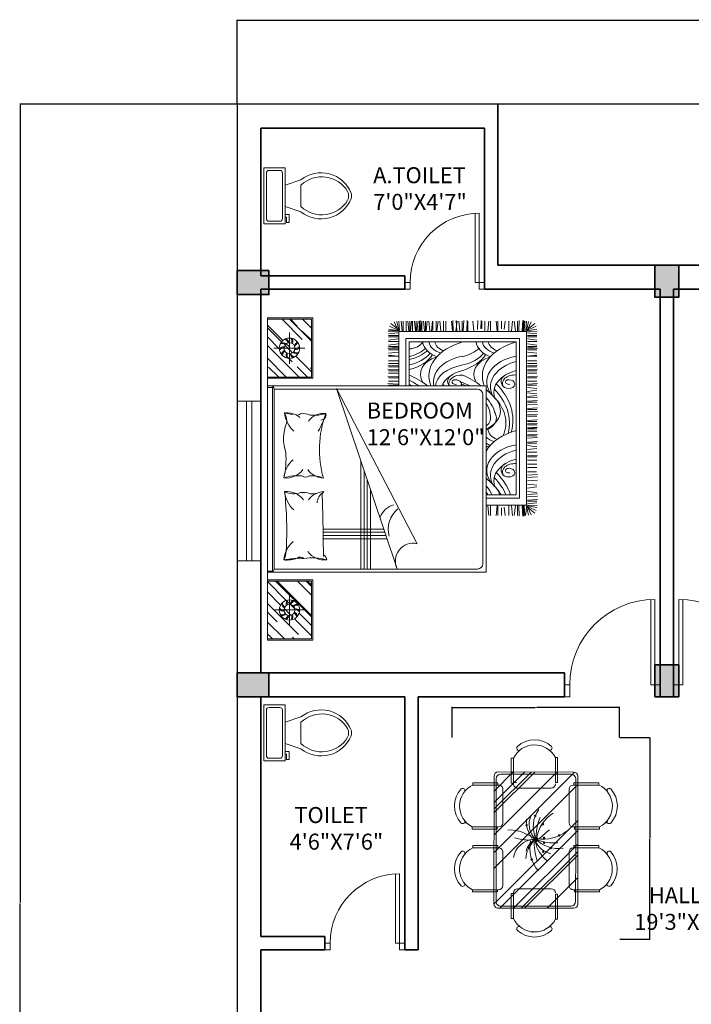
# Model space of a CAD drawing. Units: inches. Extents: x 1602 to 2642, y 1463 to 2270.
# Tile 2 of 5: x 1602 to 1854, y 1763 to 2132. Entities that reach past the tile are written whole.
import ezdxf

# ---------------------------------------------------------------- set-up
doc = ezdxf.new("R2010")
doc.units = ezdxf.units.IN
for name, color, linetype, lineweight in [('A-ANNO-DIMS', 2, 'Continuous', 18), ('A-AREA-IDEN', 7, 'Continuous', 18), ('A-COLS', 7, 'Continuous', 35), ('A-DOOR', 3, 'Continuous', 18), ('A-FLOR-FIXT', 8, 'Continuous', 18), ('A-FURN', 8, 'Continuous', 13), ('A-GLAZ', 4, 'Continuous', 18), ('A-WALL', 7, 'Continuous', 35), ('C-PROP', 7, 'Continuous', 25)]:
    doc.layers.add(name, color=color, linetype=linetype, lineweight=lineweight)
doc.styles.get("Standard").update_dxf_attribs({"font": 'arial.ttf'})
doc.dimstyles.get("Standard").update_dxf_attribs({"dimtxt": 0.18, "dimasz": 0.18, "dimexe": 0.18, "dimexo": 0.0625, "dimgap": 0.09, "dimtad": 0, "dimtih": 1, "dimtoh": 1, "dimdec": 4, "dimzin": 0, "dimdsep": 46, "dimtxsty": 'Standard', "dimcen": 0.09, "dimadec": 0, "dimazin": 0, "dimtfac": 1, "dimtdec": 4, "dimtofl": 0, "dimtmove": 0, "dimatfit": 3, "dimfxl": 1, "dimtolj": 1, "dimtzin": 0, "dimarcsym": 0})

# ---------------------------------------------------------------- blocks, each defined once
blk = doc.blocks.new('*U3')
for p, q in [((9.5, -6), (9.5, -2)), ((-10, -8.5), (-8, -8.5)), ((-10, -9.5), (-10, -8.5)), ((-7, -9.5), (-10, -9.5)), ((-8, -8.5), (-8, -8)), ((-7, -8), (-7, -9.5)), ((-4, -8), (-6, -14)), ((4, -8), (6, -14)), ((4, -14), (-4, -14))]:
    blk.add_line(p, q)
blk.add_lwpolyline([(10.5, -8), (10.5, 0), (-10.5, 0), (-10.5, -8)], close=True)
for points in [[(-9.5, -2), (-9.5, -6)], [(8.5, -1), (-8.5, -1)], [(-8.5, -7), (8.5, -7)]]:
    blk.add_lwpolyline(points)
for centre, radius, start, end in [((-8.62, -1.88), 0.884, 81.8699, 188.1301), ((8.62, -1.88), 0.884, 351.8699, 98.1301), ((-8.62, -6.12), 0.884, 171.8699, 278.1301), ((8.62, -6.12), 0.884, 261.8699, 8.1301), ((3.52, -21.58), 12.17, 141.4691, 247.9714), ((4.2, -21.82), 11.33, 136.3677, 238.9468), ((-3.52, -21.58), 12.17, 292.0284, 38.5307), ((-4.2, -21.82), 11.33, 301.053, 43.6321), ((0, -27.88), 4, 245.7318, 294.2682), ((0, -29), 4, 254.8605, 285.1395)]:
    blk.add_arc(centre, radius, start, end)
blk = doc.blocks.new('A$C6327331B')
for p, q in [((790.8, 678.3), (790.8, 696.4)), ((790.8, 678.3), (790.8, 696.4)), ((1381.3, 692.8), (1381.3, 686.2)), ((1381.3, 692.8), (1381.3, 686.2)), ((410.1, 615.8), (410, 377)), ((410.1, 615.8), (410, 377)), ((431.6, 615.8), (410.1, 615.8)), ((431.6, 615.8), (410.1, 615.8)), ((431.4, 376.9), (431.6, 615.8)), ((431.4, 376.9), (431.6, 615.8)), ((431.5, 571.8), (431.4, 370.8)), ((431.5, 571.8), (431.4, 370.8)), ((831.4, 382.9), (831.6, 621.7)), ((831.4, 382.9), (831.6, 621.7)), ((831.4, 370.6), (831.5, 571.6)), ((831.4, 370.6), (831.5, 571.6)), ((831.6, 621.7), (853, 621.7)), ((831.6, 621.7), (853, 621.7)), ((853, 621.7), (852.9, 382.9)), ((853, 621.7), (852.9, 382.9)), ((1009.3, 615.5), (1009.2, 376.7)), ((1009.3, 615.5), (1009.2, 376.7)), ((1030.7, 615.5), (1009.3, 615.5)), ((1030.7, 615.5), (1009.3, 615.5)), ((1030.6, 376.6), (1030.7, 615.5)), ((1030.6, 376.6), (1030.7, 615.5)), ((1030.7, 571.5), (1030.6, 370.5)), ((1030.7, 571.5), (1030.6, 370.5)), ((1430.6, 382.6), (1430.7, 621.4)), ((1430.6, 382.6), (1430.7, 621.4)), ((1430.6, 370.3), (1430.7, 571.3)), ((1430.6, 370.3), (1430.7, 571.3)), ((1430.7, 621.4), (1452.2, 621.4)), ((1430.7, 621.4), (1452.2, 621.4)), ((1452.2, 621.4), (1452, 382.6)), ((1452.2, 621.4), (1452, 382.6)), ((1075.9, -386.3), (308.5, 383.1)), ((1075.9, -386.3), (308.5, 383.1)), ((347.5, 414), (831.5, 413.8)), ((347.5, 414), (831.5, 413.8)), ((372.5, 394), (831.4, 393.8)), ((372.5, 394), (1009.2, 393.7)), ((410, 377), (431.4, 376.9)), ((410, 377), (431.4, 376.9)), ((1226.3, -386.4), (428, 414)), ((1226.3, -386.4), (428, 414)), ((1567.1, -386.6), (768.8, 413.8)), ((1567.1, -386.6), (768.8, 413.8)), ((852.9, 382.9), (831.4, 382.9)), ((852.9, 382.9), (831.4, 382.9)), ((831.5, 413.8), (1567.5, 413.4)), ((1607.1, -331.3), (864.1, 413.8)), ((1607.1, -331.3), (864.1, 413.8)), ((1607.2, -200.8), (994.4, 413.7)), ((1607.2, -200.8), (994.4, 413.7)), ((1009.2, 413.7), (1567.5, 413.4)), ((1009.2, 393.7), (1542.5, 393.4)), ((1009.2, 376.7), (1030.6, 376.6)), ((1009.2, 376.7), (1030.6, 376.6)), ((1607.2, -125.5), (1069.5, 413.7)), ((1607.2, -125.5), (1069.5, 413.7)), ((1607.2, -95.4), (1099.6, 413.6)), ((1607.2, -95.4), (1099.6, 413.6)), ((1607.3, 120.5), (1315.1, 413.5)), ((1607.3, 120.5), (1315.1, 413.5)), ((1415.7, 413.4), (1415.7, 413.5)), ((1415.7, 413.4), (1415.7, 413.5)), ((1452, 382.6), (1430.6, 382.6)), ((1452, 382.6), (1430.6, 382.6)), ((307.1, -346), (307.5, 374)), ((307.1, -346), (307.5, 374)), ((327.1, -321), (327.5, 349)), ((471.4, 330.8), (791.4, 330.6)), ((471.4, 330.8), (791.4, 330.6)), ((1070.6, 330.5), (1390.6, 330.3)), ((1070.6, 330.5), (1390.6, 330.3)), ((1587.5, 348.4), (1587.1, -321.6)), ((1607.5, 373.4), (1607.1, -346.6)), ((1607.5, 373.4), (1607.1, -346.6)), ((169.9, 221.5), (408.7, 221.6)), ((169.9, 221.5), (408.7, 221.6)), ((169.9, 200.1), (169.9, 221.5)), ((169.9, 200.1), (169.9, 221.5)), ((408.7, 200.2), (169.9, 200.1)), ((408.7, 200.2), (169.9, 200.1)), ((905.5, -386.3), (307.4, 213.5)), ((905.5, -386.3), (307.4, 213.5)), ((408.7, 221.6), (408.7, 200.2)), ((408.7, 221.6), (408.7, 200.2)), ((1473.3, 221.6), (1473.3, 200.2)), ((1473.3, 221.6), (1473.3, 200.2)), ((1712.1, 221.5), (1473.3, 221.6)), ((1712.1, 221.5), (1473.3, 221.6)), ((1473.3, 200.2), (1712.1, 200.1)), ((1473.3, 200.2), (1712.1, 200.1)), ((1712.1, 200.1), (1712.1, 221.5)), ((1712.1, 200.1), (1712.1, 221.5)), ((461.2, -159.8), (461, 160.2)), ((461.2, -159.8), (461, 160.2)), ((1420.8, -159.8), (1420.9, 160.2)), ((1420.8, -159.8), (1420.9, 160.2)), ((695.1, -386.2), (307.3, 2.7)), ((695.1, -386.2), (307.3, 2.7)), ((44.6, -20.2), (44.5, -20.1)), ((44.6, -20.2), (44.5, -20.1)), ((599.8, -386.1), (307.2, -92.7)), ((599.8, -386.1), (307.2, -92.7)), ((660, -386.1), (307.3, -32.5)), ((660, -386.1), (307.3, -32.5)), ((1837.4, -20.2), (1837.5, -20.1)), ((1837.4, -20.2), (1837.5, -20.1)), ((408.7, -193.6), (408.7, -172.1)), ((408.7, -193.6), (408.7, -172.1)), ((415.1, -199.8), (176.2, -199.9)), ((415.1, -199.8), (176.2, -199.9)), ((176.2, -199.9), (176.2, -221.3)), ((176.2, -199.9), (176.2, -221.3)), ((176.2, -221.3), (415.1, -221.2)), ((176.2, -221.3), (415.1, -221.2)), ((220.2, -199.9), (421.2, -199.8)), ((220.2, -199.9), (421.2, -199.8)), ((489.6, -386), (307.2, -203.2)), ((489.6, -386), (307.2, -203.2)), ((415.1, -221.2), (415.1, -199.8)), ((415.1, -221.2), (415.1, -199.8)), ((1661.8, -199.9), (1460.8, -199.8)), ((1661.8, -199.9), (1460.8, -199.8)), ((1466.9, -221.2), (1466.9, -199.8)), ((1466.9, -221.2), (1466.9, -199.8)), ((1466.9, -199.8), (1705.7, -199.9)), ((1466.9, -199.8), (1705.7, -199.9)), ((1705.7, -221.3), (1466.9, -221.2)), ((1705.7, -221.3), (1466.9, -221.2)), ((1705.7, -199.9), (1705.7, -221.3)), ((1705.7, -199.9), (1705.7, -221.3)), ((1542.1, -366.6), (372.1, -366)), ((410.1, -587.7), (410, -348.9)), ((410.1, -587.7), (410, -348.9)), ((410, -348.9), (431.4, -348.9)), ((410, -348.9), (431.4, -348.9)), ((431.5, -543.7), (431.4, -342.7)), ((431.5, -543.7), (431.4, -342.7)), ((431.4, -348.9), (431.6, -587.7)), ((431.4, -348.9), (431.6, -587.7)), ((471.4, -302.7), (791.4, -302.5)), ((471.4, -302.7), (791.4, -302.5)), ((831.4, -342.5), (831.5, -543.5)), ((831.4, -342.5), (831.5, -543.5)), ((831.4, -354.8), (831.6, -593.6)), ((831.4, -354.8), (831.6, -593.6)), ((852.9, -354.8), (831.4, -354.8)), ((852.9, -354.8), (831.4, -354.8)), ((853, -593.6), (852.9, -354.8)), ((853, -593.6), (852.9, -354.8)), ((1009.2, -348.6), (1030.6, -348.5)), ((1009.2, -348.6), (1030.6, -348.5)), ((1009.3, -587.4), (1009.2, -348.6)), ((1009.3, -587.4), (1009.2, -348.6)), ((1030.7, -543.4), (1030.6, -342.4)), ((1030.7, -543.4), (1030.6, -342.4)), ((1030.6, -348.5), (1030.7, -587.4)), ((1030.6, -348.5), (1030.7, -587.4)), ((1070.6, -302.4), (1390.6, -302.2)), ((1070.6, -302.4), (1390.6, -302.2)), ((1430.6, -342.2), (1430.7, -543.2)), ((1430.6, -342.2), (1430.7, -543.2)), ((1430.6, -354.5), (1430.7, -593.3)), ((1430.6, -354.5), (1430.7, -593.3)), ((1452, -354.5), (1430.6, -354.5)), ((1452, -354.5), (1430.6, -354.5)), ((1452.2, -593.3), (1452, -354.5)), ((1452.2, -593.3), (1452, -354.5)), ((1567.1, -386.6), (347.1, -386)), ((1567.1, -386.6), (347.1, -386)), ((831.5, -385.7), (864.1, -385.7)), ((831.5, -385.7), (864.1, -385.7)), ((1415.7, -385.3), (1415.7, -385.4)), ((1415.7, -385.3), (1415.7, -385.4)), ((431.6, -587.7), (410.1, -587.7)), ((431.6, -587.7), (410.1, -587.7)), ((790.8, -650.2), (790.8, -668.4)), ((790.8, -650.2), (790.8, -668.4)), ((831.6, -593.6), (853, -593.6)), ((831.6, -593.6), (853, -593.6)), ((1030.7, -587.4), (1009.3, -587.4)), ((1030.7, -587.4), (1009.3, -587.4)), ((1430.7, -593.3), (1452.2, -593.3)), ((1430.7, -593.3), (1452.2, -593.3)), ((1381.3, -664.7), (1381.3, -658.1)), ((1381.3, -664.7), (1381.3, -658.1))]:
    blk.add_line(p, q)
for centre, radius, start, end in [((631.5, 550.5), 241.3, 47.46915, 132.47205), ((631.5, 550.5), 241.3, 47.46915, 132.47205), ((1230.7, 550.2), 241.3, 47.46915, 132.47205), ((1230.7, 550.2), 241.3, 47.46915, 132.47205), ((633, 521.6), 222.4, 26.76564, 154.93691), ((633, 521.6), 222.4, 26.76564, 154.93691), ((484.3, 714.2), 21.2, 137.64965, 300.34124), ((484.3, 714.2), 21.2, 137.64965, 300.34124), ((779, 714), 21.2, 239.59996, 42.29154), ((779, 714), 21.2, 239.59996, 42.29154), ((1232.2, 521.3), 222.4, 84.42654, 154.93691), ((1232.2, 521.3), 222.4, 84.42654, 154.93691), ((1083.4, 713.9), 21.2, 137.64965, 300.34124), ((1083.4, 713.9), 21.2, 137.64965, 300.34124), ((1232.2, 521.3), 222.4, 26.76564, 84.42654), ((1232.2, 521.3), 222.4, 26.76564, 84.42654), ((1378.1, 713.7), 21.2, 239.59996, 42.29154), ((1378.1, 713.7), 21.2, 239.59996, 42.29154), ((347.5, 374), 40, 89.9706, 179.9706), ((347.5, 374), 40, 89.9706, 179.9706), ((372.5, 349), 45, 89.9706, 179.9706), ((1542.5, 348.4), 45, 359.9706, 89.9706), ((1567.5, 373.4), 40, 359.9706, 89.9706), ((1567.5, 373.4), 40, 359.9706, 89.9706), ((471.4, 370.8), 40, 179.9706, 269.9706), ((471.4, 370.8), 40, 179.9706, 269.9706), ((791.4, 370.6), 40, 269.9706, 359.9706), ((791.4, 370.6), 40, 269.9706, 359.9706), ((574.1, 79.9), 374.6, 351.24958, 38.23328), ((1070.6, 370.5), 40, 179.9706, 269.9706), ((1070.6, 370.5), 40, 179.9706, 269.9706), ((1390.6, 370.3), 40, 269.9706, 359.9706), ((1390.6, 370.3), 40, 269.9706, 359.9706), ((270.2, 1.6), 222.4, 116.82445, 244.99571), ((270.2, 1.6), 222.4, 116.82445, 244.99571), ((421, 160.2), 40, 0.0294, 90.0294), ((421, 160.2), 40, 0.0294, 90.0294), ((912.6, 235.7), 6.91, 0, 180), ((912.6, 235.7), 6.91, 180, 0), ((737.8, 225), 299.2, 314.48606, 9.37622), ((586.4, 182.9), 398.1, 335.08876, 5.96372), ((1460.9, 160.2), 40, 89.9706, 179.9706), ((1460.9, 160.2), 40, 89.9706, 179.9706), ((1611.7, 1.6), 222.4, 295.00429, 63.17555), ((1611.7, 1.6), 222.4, 295.00429, 63.17555), ((241.3, 0.1), 241.3, 137.52795, 222.53085), ((77.6, 147.4), 21.2, 329.65876, 132.35035), ((77.6, 147.4), 21.2, 329.65876, 132.35035), ((983.2, 350.8), 331, 211.31505, 262.13779), ((2460.3, 1443.6), 2062.1, 219.04877, 222.6799), ((934.8, 91.3), 6.91, 0, 180), ((873.8, 207.8), 219.3, 294.09558, 346.29534), ((897.1, 334.6), 335.6, 283.04524, 319.77663), ((982.3, 91.3), 6.91, 0, 180), ((1033, 155.9), 6.91, 0, 180), ((1033, 155.9), 6.91, 180, 0), ((1804.4, 147.4), 21.2, 47.64965, 210.34124), ((1804.4, 147.4), 21.2, 47.64965, 210.34124), ((1640.7, 0.1), 241.3, 317.46915, 42.47205), ((1640.7, 0.1), 241.3, 317.46915, 42.47205), ((826.9, 258.5), 270.1, 233.32313, 295.76326), ((725.8, 7.7), 6.91, 0, 180), ((725.8, 7.7), 6.91, 180, 0), ((807.8, 143), 194.5, 242.99086, 315.91017), ((985.1, 750.7), 739.8, 250.5249, 267.82437), ((805, 79.9), 6.91, 0, 180), ((805, 79.9), 6.91, 180, 0), ((1747.6, -469.5), 933.6, 148.98728, 160.36101), ((931.7, 11.5), 6.91, 0, 180), ((931.7, 11.5), 6.91, 180, 0), ((934.8, 91.3), 6.91, 180, 0), ((944.3, 26.7), 6.91, 0, 180), ((944.3, 26.7), 6.91, 180, 0), ((947.5, 3.9), 6.91, 0, 180), ((947.5, 3.9), 6.91, 180, 0), ((970.7, 574.8), 578.8, 268.32856, 288.729), ((966.5, 15.3), 6.91, 0, 180), ((966.5, 15.3), 6.91, 180, 0), ((1030.3, 292.7), 337.4, 258.55155, 310.98153), ((982.3, 91.3), 6.91, 180, 0), ((1067.8, 83.7), 6.91, 0, 180), ((1067.8, 83.7), 6.91, 180, 0), ((776.7, 191.6), 268.2, 265.87406, 306.95584), ((814.5, -75.9), 6.91, 0, 180), ((814.5, -75.9), 6.91, 180, 0), ((392.7, -33), 564.4, 343.85612, 359.11051), ((953.8, -11.3), 6.91, 0, 180), ((953.8, -11.3), 6.91, 180, 0), ((1167.7, 15.7), 221.9, 186.99045, 258.02836), ((1090.6, 62.7), 145.4, 208.89012, 258.45792), ((1166.2, 212.9), 298.2, 228.7581, 263.8624), ((995, -34.1), 6.91, 0, 180), ((995, -34.1), 6.91, 180, 0), ((1026.7, -60.7), 6.91, 0, 180), ((1026.7, -60.7), 6.91, 180, 0), ((1143.8, -26.5), 6.91, 0, 180), ((1143.8, -26.5), 6.91, 180, 0), ((79, -146.7), 22.5, 226.37763, 29.88821), ((79, -146.7), 22.5, 226.37763, 29.88821), ((421.2, -159.8), 40, 270.0294, 0.0294), ((421.2, -159.8), 40, 270.0294, 0.0294), ((1112.9, -226), 252.6, 162.94564, 186.48138), ((1460.8, -159.8), 40, 179.9706, 269.9706), ((1460.8, -159.8), 40, 179.9706, 269.9706), ((1803, -146.7), 22.5, 150.11179, 313.62237), ((1803, -146.7), 22.5, 150.11179, 313.62237), ((347.1, -346), 40, 179.9706, 269.9706), ((347.1, -346), 40, 179.9706, 269.9706), ((372.1, -321), 45, 179.9706, 269.9706), ((471.4, -342.7), 40, 90.0294, 180.0294), ((471.4, -342.7), 40, 90.0294, 180.0294), ((791.4, -342.5), 40, 0.0294, 90.0294), ((791.4, -342.5), 40, 0.0294, 90.0294), ((1070.6, -342.4), 40, 90.0294, 180.0294), ((1070.6, -342.4), 40, 90.0294, 180.0294), ((1390.6, -342.2), 40, 0.0294, 90.0294), ((1390.6, -342.2), 40, 0.0294, 90.0294), ((1542.1, -321.6), 45, 269.9706, 359.9706), ((1567.1, -346.6), 40, 269.9706, 359.9706), ((1567.1, -346.6), 40, 269.9706, 359.9706), ((633, -493.5), 222.4, 205.06309, 333.23436), ((633, -493.5), 222.4, 205.06309, 333.23436), ((1232.2, -493.2), 222.4, 205.06309, 275.57346), ((1232.2, -493.2), 222.4, 205.06309, 275.57346), ((1232.2, -493.2), 222.4, 275.57346, 333.23436), ((1232.2, -493.2), 222.4, 275.57346, 333.23436), ((484.3, -686.1), 21.2, 59.65876, 222.35035), ((484.3, -686.1), 21.2, 59.65876, 222.35035), ((631.5, -522.4), 241.3, 227.52795, 312.53085), ((631.5, -522.4), 241.3, 227.52795, 312.53085), ((779, -686), 21.2, 317.70846, 120.40004), ((779, -686), 21.2, 317.70846, 120.40004), ((1083.4, -685.8), 21.2, 59.65876, 222.35035), ((1083.4, -685.8), 21.2, 59.65876, 222.35035), ((1230.7, -522.1), 241.3, 227.52795, 312.53085), ((1230.7, -522.1), 241.3, 227.52795, 312.53085), ((1378.1, -685.6), 21.2, 317.70846, 120.40004), ((1378.1, -685.6), 21.2, 317.70846, 120.40004)]:
    blk.add_arc(centre, radius, start, end)
at = {"width": 0.8, "flags": 9}
for tag in ['XSIZE', 'YSIZE']:
    blk.add_attdef(tag, (945.2, 11.4), '', height=0.23, rotation=180, dxfattribs=at)
blk = doc.blocks.new('A$C64B41DC1')
for p, q in [((0, 2.5079), (2.9903, 2.5079)), ((0, 2.0879), (0, 2.5079)), ((0.012, 2.4618), (0.0581, 2.5079)), ((0.012, 2.3515), (0.1684, 2.5079)), ((0.012, 2.0999), (0.012, 2.5079)), ((0.0543, 2.2213), (0.3409, 2.5079)), ((0.1689, 2.4179), (0.2589, 2.5079)), ((0.3265, 2.386), (0.4484, 2.5079)), ((0.3699, 2.3332), (0.5445, 2.5079)), ((0.548, 2.5079), (0.548, 2.0999)), ((0.56, 2.5079), (0.56, 2.0879)), ((0.6301, 2.5079), (0.6301, 0.4779)), ((0.6401, 2.461), (0.6401, 2.5079)), ((0.6401, 2.5079), (2.344, 2.5079)), ((2.344, 2.5079), (2.3601, 2.5079)), ((2.344, 2.5079), (2.344, 2.461)), ((2.3601, 2.5079), (2.3601, 2.4761)), ((2.3601, 0.4779), (2.3601, 2.5079)), ((2.4303, 2.5079), (2.4303, 2.0879)), ((2.4423, 2.5079), (2.4423, 2.0999)), ((2.4423, 2.3333), (2.6169, 2.5079)), ((2.4423, 2.2145), (2.7357, 2.5079)), ((2.4423, 2.404), (2.5354, 2.4971)), ((2.705, 2.398), (2.8149, 2.5079)), ((2.7691, 2.3772), (2.8998, 2.5079)), ((2.7819, 2.3646), (2.9252, 2.5079)), ((2.9783, 2.0999), (2.9783, 2.5079)), ((2.9903, 2.0879), (2.9903, 2.5079)), ((0.2157, 2.0999), (0.548, 2.4322)), ((0.2299, 2.0999), (0.548, 2.418)), ((0.2804, 2.1597), (0.2804, 2.4481)), ((2.344, 2.461), (0.6401, 2.461)), ((0.6601, 2.4461), (1.4951, 2.4461)), ((0.6601, 2.4461), (0.6601, 0.5579)), ((1.4951, 2.4461), (0.6697, 2.4461)), ((2.3301, 2.4461), (1.4951, 2.4461)), ((2.3301, 0.5579), (2.3301, 2.4461)), ((2.7099, 2.1597), (2.7099, 2.4481)), ((0.1362, 2.3039), (0.4246, 2.3039)), ((0.2311, 2.2906), (0.2937, 2.3532)), ((0.2905, 2.2539), (0.3304, 2.2938)), ((0.3405, 2.3039), (0.3605, 2.3238)), ((2.8541, 2.3039), (2.5657, 2.3039)), ((2.5849, 2.2779), (2.6158, 2.3088)), ((2.6158, 2.3088), (2.6313, 2.3243)), ((2.6674, 2.2756), (2.7382, 2.3464)), ((2.7249, 2.3076), (2.7512, 2.3339)), ((2.7746, 2.0999), (2.9783, 2.3036)), ((2.7914, 2.1846), (2.9783, 2.3715)), ((2.9144, 2.2312), (2.9783, 2.2951)), ((0.012, 2.261), (0.0275, 2.2765)), ((0.0404, 2.0999), (0.1982, 2.2578)), ((0.1365, 2.0999), (0.251, 2.2144)), ((0.4194, 2.0999), (0.548, 2.2285)), ((2.4423, 2.1353), (2.5382, 2.2312)), ((2.4918, 2.0999), (2.6366, 2.2447)), ((0.4986, 2.0999), (0.548, 2.1493)), ((0.5127, 2.0999), (0.548, 2.1352)), ((2.5172, 2.0999), (2.5269, 2.1096)), ((2.7831, 2.0999), (2.8678, 2.1846)), ((2.8962, 2.0999), (2.9783, 2.182)), ((0.56, 2.0879), (0, 2.0879)), ((0.548, 2.0999), (0.012, 2.0999)), ((2.4303, 2.0879), (2.9903, 2.0879)), ((2.4423, 2.0999), (2.9783, 2.0999)), ((0.9415, 1.9902), (0.9415, 1.3975)), ((0.9715, 1.9906), (0.9715, 1.4076)), ((1.0015, 1.991), (1.0015, 1.4177)), ((1.0315, 1.9916), (1.0315, 1.4279)), ((2.3349, 1.8678), (0.6613, 1.3029)), ((0.8956, 1.1191), (2.3349, 1.8678)), ((1.6636, 1.6412), (0.6601, 1.6412)), ((1.5748, 1.6112), (0.6601, 1.6112)), ((2.3665, 1.295), (2.3665, 1.3839)), ((2.377, 1.295), (2.3822, 1.3891)), ((2.4032, 1.295), (2.4032, 1.3839)), ((2.4346, 1.295), (2.4346, 1.3839)), ((2.4451, 1.295), (2.4503, 1.3891)), ((2.4774, 1.2957), (2.4774, 1.3837)), ((2.5, 1.295), (2.5, 1.3839)), ((2.5105, 1.295), (2.5157, 1.3891)), ((2.5367, 1.295), (2.5367, 1.3839)), ((2.5471, 1.295), (2.5524, 1.3891)), ((2.5681, 1.295), (2.5681, 1.3839)), ((2.5918, 1.295), (2.5918, 1.3839)), ((2.6346, 1.2957), (2.6346, 1.3837)), ((2.6362, 1.2957), (2.6467, 1.3839)), ((2.6729, 1.295), (2.6624, 1.3839)), ((2.6938, 1.295), (2.6938, 1.3839)), ((2.7043, 1.295), (2.7095, 1.3891)), ((2.7127, 1.2957), (2.7232, 1.3839)), ((2.7253, 1.295), (2.7253, 1.3839)), ((2.7494, 1.295), (2.7389, 1.3839)), ((2.7718, 1.295), (2.7718, 1.3839)), ((2.7959, 1.295), (2.7854, 1.3839)), ((2.8146, 1.2957), (2.8146, 1.3837)), ((2.8146, 1.2957), (2.8146, 1.3837)), ((2.8282, 1.295), (2.8282, 1.3839)), ((2.8282, 1.295), (2.8282, 1.3839)), ((2.8523, 1.295), (2.8418, 1.3839)), ((2.8523, 1.295), (2.8418, 1.3839)), ((2.8653, 1.2966), (2.8688, 1.3861)), ((2.8711, 1.2957), (2.8711, 1.3837)), ((2.8711, 1.2957), (2.8875, 1.3822)), ((2.8765, 1.2958), (2.9132, 1.3758)), ((2.3601, 1.2873), (2.8639, 1.2873)), ((2.8639, 1.2873), (2.8639, 0.1018)), ((2.8713, 1.2927), (2.954, 1.3315)), ((2.8717, 1.2884), (2.9588, 1.3058)), ((2.8744, 1.2817), (2.9603, 1.2869)), ((2.8893, 1.3011), (2.9394, 1.3636)), ((2.3601, 1.2233), (2.7999, 1.2233)), ((2.3601, 1.1913), (2.7679, 1.1912)), ((2.7679, 1.1912), (2.7679, 0.1978)), ((2.7999, 1.2233), (2.7999, 0.1658)), ((2.8716, 1.2565), (2.9605, 1.2669)), ((2.8716, 1.2212), (2.9605, 1.2212)), ((2.8716, 1.1947), (2.9605, 1.2052)), ((2.8723, 1.2489), (2.9603, 1.2489)), ((2.8716, 1.181), (2.9605, 1.1705)), ((2.8716, 1.1595), (2.9605, 1.1595)), ((2.8716, 1.133), (2.9605, 1.1435)), ((2.8716, 1.1193), (2.9605, 1.1088)), ((2.8716, 1.1035), (2.9605, 1.093)), ((2.8723, 1.1872), (2.9603, 1.1872)), ((2.8723, 1.1255), (2.9603, 1.1255)), ((2.8716, 1.0965), (2.9605, 1.0965)), ((2.8716, 1.086), (2.9657, 1.0913)), ((2.8716, 1.0756), (2.9605, 1.0756)), ((2.8716, 1.0491), (2.9605, 1.0596)), ((2.8716, 1.0354), (2.9605, 1.0249)), ((2.8723, 1.0858), (2.9605, 1.0753)), ((2.8723, 1.0416), (2.9603, 1.0416)), ((2.8723, 0.9987), (2.9605, 1.0092)), ((2.8716, 0.9346), (2.9605, 0.9241)), ((2.8723, 0.985), (2.9605, 0.9745)), ((2.8723, 0.9735), (2.9603, 0.9735)), ((2.8723, 0.9408), (2.9603, 0.9408)), ((2.8723, 0.8979), (2.9605, 0.9084)), ((2.8723, 0.8726), (2.9603, 0.8726)), ((2.8723, 0.8505), (2.9603, 0.8505)), ((2.8716, 0.7885), (2.9605, 0.799)), ((2.8716, 0.7818), (2.9657, 0.787)), ((2.8716, 0.7503), (2.9657, 0.7556)), ((2.8723, 0.7571), (2.9605, 0.7466)), ((2.8716, 0.7204), (2.9605, 0.7309)), ((2.8716, 0.6995), (2.9605, 0.6995)), ((2.8716, 0.689), (2.9657, 0.6838)), ((2.8716, 0.6576), (2.9657, 0.6523)), ((2.8716, 0.6471), (2.9605, 0.6471)), ((2.8716, 0.5903), (2.9605, 0.6007)), ((2.882, 0.5582), (2.9657, 0.5536)), ((0.6301, 0.4779), (2.3601, 0.4779)), ((0.7101, 0.5079), (2.2801, 0.5079)), ((1.2465, 0.4625), (1.1576, 0.452)), ((1.2542, 0.1018), (1.2542, 0.4779)), ((1.3182, 0.1658), (1.3182, 0.4779)), ((1.3502, 0.1978), (1.3502, 0.4779)), ((2.8716, 0.4877), (2.9603, 0.4877)), ((2.8716, 0.4625), (2.9605, 0.452)), ((2.8909, 0.5263), (2.9657, 0.5222)), ((2.8928, 0.5169), (2.9605, 0.5169)), ((1.2465, 0.3746), (1.1576, 0.3851)), ((1.2465, 0.4365), (1.1577, 0.4365)), ((1.2465, 0.3684), (1.1577, 0.3684)), ((2.8716, 0.4365), (2.9603, 0.4365)), ((2.8716, 0.3746), (2.9605, 0.3851)), ((2.8716, 0.3684), (2.9603, 0.3684)), ((1.2355, 0.3092), (1.1576, 0.3)), ((1.2285, 0.3357), (1.1577, 0.3357)), ((2.8826, 0.3092), (2.9605, 0.3)), ((2.8896, 0.3357), (2.9603, 0.3357)), ((1.2457, 0.2423), (1.1576, 0.2319)), ((1.2465, 0.2057), (1.1576, 0.2161)), ((1.2465, 0.1847), (1.1576, 0.1847)), ((1.2457, 0.2676), (1.1577, 0.2676)), ((2.7679, 0.1978), (1.3502, 0.1978)), ((2.8716, 0.2057), (2.9605, 0.2161)), ((2.8716, 0.1847), (2.9605, 0.1847)), ((2.8723, 0.2676), (2.9603, 0.2676)), ((2.8723, 0.2423), (2.9605, 0.2319)), ((1.2465, 0.1742), (1.1524, 0.169)), ((1.2465, 0.1428), (1.1524, 0.1376)), ((1.2465, 0.1334), (1.1524, 0.1281)), ((1.2465, 0.1323), (1.1576, 0.1323)), ((1.2465, 0.1323), (1.1576, 0.1323)), ((1.2465, 0.1), (1.1576, 0.1105)), ((1.2465, 0.1229), (1.1588, 0.1168)), ((1.2464, 0.1007), (1.1592, 0.0833)), ((1.2468, 0.0964), (1.1641, 0.0576)), ((1.2415, 0.0933), (1.2049, 0.0133)), ((1.247, 0.0934), (1.2306, 0.0069)), ((1.2527, 0.0925), (1.2493, 0.003)), ((2.8639, 0.1018), (1.2542, 0.1018)), ((1.2658, 0.0941), (1.2762, 0.0052)), ((1.2899, 0.0941), (1.2899, 0.0052)), ((1.2999, 0.0941), (1.3051, 0)), ((2.7999, 0.1658), (1.3182, 0.1658)), ((1.3313, 0.0941), (1.3365, 0)), ((1.3523, 0.0941), (1.3575, 0)), ((1.3804, 0.0941), (1.3699, 0.0052)), ((1.4119, 0.0934), (1.4223, 0.0052)), ((1.4485, 0.0941), (1.438, 0.0052)), ((1.48, 0.0941), (1.4852, 0)), ((1.5114, 0.0941), (1.5166, 0)), ((1.5323, 0.0941), (1.5376, 0)), ((1.5638, 0.0941), (1.5638, 0.0105)), ((1.6021, 0.0941), (1.6021, 0.0052)), ((1.6336, 0.0941), (1.6336, 0.0052)), ((1.6702, 0.0941), (1.6702, 0.0052)), ((1.7017, 0.0941), (1.7017, 0.0052)), ((1.7122, 0.0941), (1.7174, 0)), ((1.7445, 0.0934), (1.7445, 0.0054)), ((1.7698, 0.0934), (1.7803, 0.0052)), ((1.8065, 0.0941), (1.796, 0.0052)), ((1.8274, 0.0941), (1.8274, 0.0052)), ((1.8379, 0.0941), (1.8431, 0)), ((1.8746, 0.0941), (1.8798, 0)), ((1.8955, 0.0941), (1.8955, 0.0052)), ((1.906, 0.0941), (1.9113, 0)), ((1.9384, 0.0934), (1.9384, 0.0054)), ((1.9609, 0.0941), (1.9609, 0.0052)), ((1.9636, 0.0934), (1.9741, 0.0052)), ((1.9714, 0.0941), (1.9766, 0)), ((1.9976, 0.0941), (1.9976, 0.0052)), ((2.0081, 0.0941), (2.0133, 0)), ((2.029, 0.0941), (2.029, 0.0052)), ((2.0395, 0.0941), (2.0447, 0)), ((2.0797, 0.0941), (2.0797, 0.0052)), ((2.0902, 0.0941), (2.0954, 0)), ((2.1216, 0.0941), (2.1269, 0)), ((2.1412, 0.0941), (2.1412, 0.0052)), ((2.1517, 0.0941), (2.1569, 0)), ((2.1831, 0.0941), (2.1884, 0)), ((2.2093, 0.0941), (2.2093, 0.0052)), ((2.2198, 0.0941), (2.225, 0)), ((2.2512, 0.0941), (2.2565, 0)), ((2.2603, 0.0934), (2.2707, 0.0052)), ((2.2969, 0.0941), (2.2864, 0.0052)), ((2.3089, 0.0934), (2.3193, 0.0052)), ((2.3455, 0.0941), (2.3351, 0.0052)), ((2.3665, 0.0941), (2.3665, 0.0052)), ((2.377, 0.0941), (2.3822, 0)), ((2.4032, 0.0941), (2.4032, 0.0052)), ((2.4346, 0.0941), (2.4346, 0.0052)), ((2.4451, 0.0941), (2.4503, 0)), ((2.4774, 0.0934), (2.4774, 0.0054)), ((2.5, 0.0941), (2.5, 0.0052)), ((2.5105, 0.0941), (2.5157, 0)), ((2.5367, 0.0941), (2.5367, 0.0052)), ((2.5471, 0.0941), (2.5524, 0)), ((2.5681, 0.0941), (2.5681, 0.0052)), ((2.5918, 0.0941), (2.5918, 0.0052)), ((2.6346, 0.0934), (2.6346, 0.0054)), ((2.6362, 0.0934), (2.6467, 0.0052)), ((2.6729, 0.0941), (2.6624, 0.0052)), ((2.6938, 0.0941), (2.6938, 0.0052)), ((2.7043, 0.0941), (2.7095, 0)), ((2.7127, 0.0934), (2.7232, 0.0052)), ((2.7253, 0.0941), (2.7253, 0.0052)), ((2.7494, 0.0941), (2.7389, 0.0052)), ((2.7718, 0.0941), (2.7718, 0.0052)), ((2.7959, 0.0941), (2.7854, 0.0052)), ((2.8146, 0.0934), (2.8146, 0.0054)), ((2.8282, 0.0941), (2.8282, 0.0052)), ((2.8523, 0.0941), (2.8418, 0.0052)), ((2.8653, 0.0925), (2.8688, 0.003)), ((2.8711, 0.0934), (2.8875, 0.0069)), ((2.8713, 0.0964), (2.954, 0.0576)), ((2.8716, 0.1742), (2.9657, 0.169)), ((2.8716, 0.1428), (2.9657, 0.1376)), ((2.8716, 0.1334), (2.9657, 0.1281)), ((2.8716, 0.1323), (2.9605, 0.1323)), ((2.8716, 0.1229), (2.9593, 0.1168)), ((2.8717, 0.1007), (2.9588, 0.0833)), ((2.8744, 0.1074), (2.9603, 0.1022)), ((2.8765, 0.0933), (2.9132, 0.0133)), ((1.2288, 0.088), (1.1787, 0.0255)), ((2.8893, 0.088), (2.9394, 0.0255))]:
    blk.add_line(p, q)
at = {"ltscale": 10}
for p, q in [((1.4859, 1.5812), (0.6601, 1.5812)), ((1.397, 1.5512), (0.6601, 1.5512))]:
    blk.add_line(p, q, dxfattribs=at)
for centre, radius in [((0.2804, 2.3039), 0.0942), ((2.7099, 2.3039), 0.0942), ((0.2804, 2.3039), 0.051), ((2.7099, 2.3039), 0.051)]:
    blk.add_circle(centre, radius)
for centre, radius, start, end in [((0.6601, 2.4761), 0.03, 180, 270), ((2.3301, 2.4761), 0.03, 270, 0), ((0.2887, 2.3745), 0.0605, 172.17003, 218.48975), ((0.2828, 2.3731), 0.0462, 160.30017, 220.53802), ((0.3286, 2.3561), 0.0605, 136.17003, 182.48975), ((0.3231, 2.3585), 0.0462, 124.30017, 184.53802), ((0.3501, 2.3178), 0.0605, 100.17003, 146.48975), ((2.6402, 2.3178), 0.0605, 33.51025, 79.82997), ((2.6672, 2.3585), 0.0462, 355.46198, 55.69983), ((2.6617, 2.3561), 0.0605, 357.51025, 43.82997), ((2.7075, 2.3731), 0.0462, 319.46198, 19.69983), ((2.7016, 2.3745), 0.0605, 321.51025, 7.82997), ((0.2153, 2.3276), 0.0462, 232.30017, 292.53802), ((0.2457, 2.3659), 0.0605, 208.17003, 254.48975), ((0.2417, 2.3614), 0.0462, 196.30017, 256.53802), ((0.347, 2.323), 0.0462, 88.30017, 148.53802), ((0.3449, 2.2742), 0.0605, 64.17003, 110.48975), ((0.3455, 2.2802), 0.0462, 52.30017, 112.53802), ((0.3191, 2.2464), 0.0462, 16.30017, 76.53802), ((0.3151, 2.2419), 0.0605, 28.17003, 74.48975), ((1.0526, 2.3302), 0.3085, 175.30484, 198.69419), ((-0.8702, 2.0941), 1.6364, 4.80985, 9.18918), ((0.8579, 2.6278), 0.2948, 247.51785, 264.26696), ((0.728, 2.111), 0.245, 40.4189, 85.9871), ((1.0164, 5.7096), 3.3803, 266.81337, 276.16021), ((1.3963, 2.1044), 0.245, 94.0129, 139.5811), ((1.1858, 2.3288), 0.1943, 306.5711, 5.88998), ((1.5348, 2.2652), 0.1767, 151.77364, 201.69827), ((1.6986, 2.3355), 0.1943, 174.11002, 233.4289), ((1.1481, 2.2311), 0.3783, 353.49469, 19.18669), ((1.6871, 3.192), 0.8561, 257.74383, 273.62843), ((1.4882, 2.111), 0.245, 40.4189, 85.9871), ((1.8674, 1.9709), 0.3878, 68.20259, 108.9817), ((2.1269, 2.1044), 0.245, 94.0129, 139.5811), ((2.0342, 2.4856), 0.1563, 261.59582, 298.90918), ((1.9165, 2.3288), 0.1943, 333.73715, 5.88998), ((2.6058, 2.2028), 0.517, 163.60457, 172.3273), ((2.6448, 2.2802), 0.0462, 67.46198, 127.69983), ((2.6454, 2.2742), 0.0605, 69.51025, 115.82997), ((2.6752, 2.2419), 0.0605, 105.51025, 151.82997), ((2.6712, 2.2464), 0.0462, 103.46198, 163.69983), ((2.6433, 2.323), 0.0462, 31.46198, 91.69983), ((2.775, 2.3276), 0.0462, 247.46198, 307.69983), ((2.7486, 2.3614), 0.0462, 283.46198, 343.69983), ((2.7446, 2.3659), 0.0605, 285.51025, 331.82997), ((0.2158, 2.3336), 0.0605, 244.17003, 290.48975), ((0.2138, 2.2848), 0.0462, 268.30017, 328.53802), ((0.2107, 2.29), 0.0605, 280.17003, 326.48975), ((0.2377, 2.2493), 0.0462, 304.30017, 4.53802), ((0.2322, 2.2517), 0.0605, 316.17003, 2.48975), ((0.2779, 2.2347), 0.0462, 340.30017, 40.53802), ((0.272, 2.2333), 0.0605, 352.17003, 38.48975), ((0.7274, 2.2013), 0.0446, 314.4736, 42.17134), ((-1.6008, 2.277), 2.3618, 357.39054, 358.88764), ((1.204, 2.1778), 0.1681, 337.01697, 7.53676), ((1.9165, 2.3288), 0.1943, 320.94042, 333.73715), ((2.1347, 2.2313), 0.0459, 165.35061, 223.26844), ((1.9346, 2.1778), 0.1681, 337.01697, 7.53676), ((2.7182, 2.2333), 0.0605, 141.51025, 187.82997), ((2.7123, 2.2347), 0.0462, 139.46198, 199.69983), ((2.7581, 2.2517), 0.0605, 177.51025, 223.82997), ((2.7526, 2.2493), 0.0462, 175.46198, 235.69983), ((2.7796, 2.29), 0.0605, 213.51025, 259.82997), ((2.7765, 2.2848), 0.0462, 211.46198, 271.69983), ((2.7744, 2.3336), 0.0605, 249.51025, 295.82997), ((0.9385, 1.978), 0.1943, 126.5711, 185.88998), ((0.2688, 2.0945), 0.4956, 344.0243, 8.70709), ((1.1858, 1.9714), 0.1943, 4.31813, 53.4289), ((1.5415, 2.0969), 0.1834, 175.22328, 196.23004), ((1.7059, 1.9714), 0.204, 127.11975, 175.09005), ((1.5671, 2.1546), 0.0547, 142.08329, 220.902), ((1.1965, 2.0983), 0.3299, 343.79543, 3.55541), ((1.9394, 1.991), 0.1651, 351.26213, 55.75721), ((2.4617, 2.0719), 0.3745, 173.82958, 196.4356), ((1.2687, 1.9248), 0.1223, 33.62799, 86.47438), ((1.7676, 1.0629), 0.9631, 69.65065, 105.96307), ((2.2748, 2.5795), 0.6373, 238.34989, 254.31375), ((2.0911, 2.0123), 0.0478, 179.77267, 283.80184), ((0.7417, 2.0149), 0.057, 273.47085, 328.54118), ((0.728, 2.2025), 0.245, 274.0129, 278.34166), ((0.7246, 18.8439), 16.8552, 270.17399, 272.05214), ((1.3401, 1.9404), 0.0603, 49.09906, 101.37023), ((1.0274, 1.1334), 0.2527, 40.62904, 104.37123), ((1.0747, 1.2871), 0.1871, 14.1863, 69.12121), ((0.7347, 1.1553), 0.1649, 347.31088, 116.44537), ((0.7101, 0.5579), 0.05, 180, 270), ((2.2801, 0.5579), 0.05, 270, 0)]:
    blk.add_arc(centre, radius, start, end)
for centre, major_axis, ratio, start_param, end_param in [((1.9938, 1.6262), (0, -0.7531), 0.68, 0.797284, 0.954936), ((2.0643, 1.466), (0, -0.5322), 0.68, 7.239912, 7.311536), ((1.9052, 1.7397), (0, -0.9842), 0.68, 0.74745, 0.979724), ((2.7455, 1.3081), (0, 0.3614), 0.68, 1.900046, 2.742661), ((2.7868, 1.3081), (0, 0.3614), 0.68, 1.900046, 2.614747), ((2.8372, 1.3081), (0, 0.3614), 0.68, 1.900046, 2.479658), ((2.8607, 1.3211), (0, 0.3614), 0.68, 1.938265, 2.479658), ((2.8057, 1.2079), (0, -0.1524), 0.68, 4.821745, 5.895886), ((2.4665, 0.8216), (0, -0.2664), 0.68, 2.006169, 3.565187), ((2.4513, 0.5069), (0, 0.502), 0.68, 5.095327, 6.553458), ((2.7862, 0.8069), (0, -0.2615), 0.68, 3.244645, 4.205018), ((2.7784, 0.8289), (0, -0.1802), 0.68, 3.227058, 4.318474), ((2.396, 0.6032), (0, 0.3641), 0.68, -1.3172, 0.145284), ((2.3507, 0.5642), (0.0073, 0.3819), 0.56205, -1.21172, -0.009991), ((2.7821, 0.7971), (0, -0.1589), 0.68, 3.272942, 4.229533), ((2.2964, 0.5771), (0, -0.3263), 0.68, 1.938944, 2.850232), ((2.0403, 1.6015), (0, -0.8763), 0.68, 6.849801, 6.887077), ((2.4005, 0.7132), (0, -0.1214), 0.68, 2.284368, 3.652258), ((2.3834, 0.7081), (0, 0.1147), 0.68, 4.593909, 6.585576), ((2.3774, 0.7653), (0, -0.0593), 0.68, 5.841311, 7.755362), ((2.3961, 0.7628), (0, -0.0317), 0.68, 1.462497, 5.046281), ((1.9938, 1.1295), (-0.0678, 0.7439), 0.610498, 3.917146, 4.063997), ((2.0643, 0.9693), (0, -0.5322), 0.68, 7.239912, 7.336618), ((1.9052, 1.243), (0, -0.9842), 0.68, 0.74745, 0.979724), ((2.7455, 0.8114), (-0.0599, 0.3735), 0.695517, 1.775813, 2.548612), ((2.7868, 0.8114), (0, 0.3614), 0.68, 1.900046, 2.614747), ((2.8607, 0.8243), (0, 0.3614), 0.68, 1.938265, 2.479658), ((2.4513, 0.0102), (0, 0.502), 0.68, 5.095327, 6.553458), ((2.4665, 0.3249), (0, -0.2664), 0.68, 2.006169, 3.565187), ((2.7862, 0.3102), (0, -0.2615), 0.68, 3.244645, 4.205018), ((1.242, 0.9693), (0, -0.5322), 0.68, 6.586764, 6.677612), ((1.1714, 1.1295), (-0.1157, 0.7241), 0.59432, 3.291697, 3.50733), ((1.0828, 1.243), (0, -0.9842), 0.68, 0.565948, 0.680366), ((1.5283, 0.0674), (0, -0.3703), 0.68, 1.930561, 3.464283), ((1.5736, 0.1065), (0, 0.3641), 0.68, -1.3172, 0.476403), ((1.6289, 0.0102), (0, 0.502), 0.68, 6.655152, 6.661293), ((1.6289, 0.0102), (0, 0.502), 0.68, 5.095327, 5.911219), ((1.6442, 0.3249), (0, -0.2664), 0.68, 2.006169, 2.182797), ((1.9638, 0.3102), (0, -0.2615), 0.68, 4.015924, 4.205018), ((1.956, 0.3322), (0, -0.1802), 0.68, 3.770744, 4.318474), ((1.9597, 0.3004), (0, -0.1589), 0.68, 3.14258, 4.229533), ((2.0606, 0.5616), (0, -0.1803), 0.68, 5.194792, 5.929328), ((2.0606, 0.5616), (0, -0.1803), 0.68, 5.194792, 6.723255), ((2.1315, 0.6603), (0, -0.3155), 0.68, 5.328638, 6.949396), ((2.0549, 0.5656), (0, -0.1303), 0.68, 5.450951, 6.054641), ((2.0643, 0.9693), (0, -0.5322), 0.68, 6.20013, 6.677612), ((1.9938, 1.1295), (-0.0678, 0.7439), 0.610498, 3.199135, 3.592282), ((1.9052, 1.243), (0, -0.9842), 0.68, 0.565948, 0.680366), ((2.3507, 0.0674), (0, -0.3703), 0.68, 1.930561, 3.464283), ((2.396, 0.1065), (0, 0.3641), 0.68, -1.3172, 0.476403), ((2.4513, 0.0102), (0, 0.502), 0.68, 6.655152, 6.661293), ((2.7784, 0.3322), (0, -0.1802), 0.68, 3.227058, 4.318474), ((2.7821, 0.3004), (0, -0.1589), 0.68, 3.272942, 4.229533), ((1.1933, 0.9181), (0, -0.624), 0.68, 0.378672, 0.625379), ((1.3091, 0.6603), (0, -0.3155), 0.68, 6.475719, 6.949396), ((1.1911, 1.1066), (0, 0.8458), 0.68, 3.421828, 3.728616), ((1.2179, 1.1047), (0, -0.8763), 0.68, 6.507006, 6.887077), ((1.474, 0.0804), (0, -0.3263), 0.68, 1.938944, 3.339184), ((2.0157, 0.9181), (0, -0.624), 0.68, -0.280078, 0.625379), ((2.0135, 1.1066), (0, 0.8458), 0.68, 2.978727, 3.728616), ((2.0403, 1.1047), (0, -0.8763), 0.68, 6.099302, 6.887077), ((2.2964, 0.0804), (0, -0.3263), 0.68, 1.938944, 3.339184), ((1.555, 0.2685), (0, -0.0593), 0.68, 3.732151, 7.755362), ((1.5781, 0.2165), (0, -0.1214), 0.68, 2.284368, 3.726131), ((1.561, 0.2114), (0, 0.1147), 0.68, 4.593909, 6.647252), ((1.5737, 0.2661), (0, -0.0317), 0.68, 1.462497, 5.046281), ((2.3774, 0.2685), (0, -0.0593), 0.68, 3.732151, 7.755362), ((2.4005, 0.2165), (0, -0.1214), 0.68, 2.284368, 3.726131), ((2.3834, 0.2114), (0, 0.1147), 0.68, 4.593909, 6.647252), ((2.3961, 0.2661), (0, -0.0317), 0.68, 1.462497, 5.046281)]:
    blk.add_ellipse(centre, major_axis=major_axis, ratio=ratio, start_param=start_param, end_param=end_param)
blk = doc.blocks.new('DOOR-SWING-26IN')
for p, q in [((26.5, 28.46), (26.5, 2.5)), ((28, 28.5), (28, 2.5)), ((0, 2.5), (2, 2.5)), ((2, 2.5), (2, 0)), ((28, 2.5), (26.5, 2.5)), ((30, 2.5), (28, 2.5)), ((28, 2.5), (28, 0)), ((2, 0), (0, 0)), ((28, 0), (30, 0))]:
    blk.add_line(p, q)
blk.add_arc((28, 2.5), 26, 90, 180)
blk = doc.blocks.new('DOOR-SWING-32IN')
for p, q in [((32.5, 4.5), (32.5, 36.46)), ((34, 4.5), (34, 36.5)), ((0, 4.5), (2, 4.5)), ((2, 4.5), (2, 0)), ((34, 4.5), (32.5, 4.5)), ((36, 4.5), (34, 4.5)), ((34, 4.5), (34, 0)), ((2, 0), (0, 0)), ((34, 0), (36, 0))]:
    blk.add_line(p, q)
blk.add_arc((34, 4.5), 32, 90, 180)
blk = doc.blocks.new('WIN-60IN')
for p, q in [((0, 0), (0, 9)), ((60, 0), (60, 9)), ((60, 5.5), (0, 5.5)), ((60, 3.5), (0, 3.5))]:
    blk.add_line(p, q)
blk = doc.blocks.new('COL-12X9')
h = blk.add_hatch(color=256)
h.dxf.hatch_style = 1
h.paths.add_polyline_path([(12, 0), (12, 9), (0, 9), (0, 0)])
blk.add_lwpolyline([(12, 9), (12, 0), (0, 0), (0, 9)], close=True)
blk = doc.blocks.new('*D17')
at = {"layer": 'A-ANNO-DIMS', "color": 0, "lineweight": -2, "transparency": 16777216}
for p, q in [((1827.54, 1862.9), (1839.01, 1862.9)), ((1838.83, 1862.72), (1838.83, 1825.24)), ((1838.83, 1787.39), (1838.83, 1824.87)), ((1827.54, 1787.21), (1839.01, 1787.21))]:
    blk.add_line(p, q, dxfattribs=at)
at = {"layer": 'A-ANNO-DIMS', "color": 0, "transparency": 16777216}
for points in [[(1838.8, 1862.72), (1838.86, 1862.72), (1838.83, 1862.9)], [(1838.8, 1787.39), (1838.86, 1787.39), (1838.83, 1787.21)]]:
    blk.add_solid(points, dxfattribs=at)
at = {"layer": 'Defpoints', "color": 0, "transparency": 16777216}
for p in [(1827.47, 1862.9), (1827.47, 1787.21), (1838.83, 1787.21)]:
    blk.add_point(p, dxfattribs=at)
at = {"layer": 'A-ANNO-DIMS', "color": 0, "transparency": 16777216, "insert": (1838.83, 1825.06), "char_height": 0.18, "attachment_point": 5}
blk.add_mtext('\\A1;DINING 76', dxfattribs=at)
blk = doc.blocks.new('*D18')
at = {"layer": 'A-ANNO-DIMS', "color": 0, "lineweight": -2, "transparency": 16777216}
for p, q in [((1764.62, 1862.97), (1764.62, 1874.44)), ((1764.8, 1874.26), (1795.83, 1874.26)), ((1827.29, 1874.26), (1796.27, 1874.26)), ((1827.47, 1862.97), (1827.47, 1874.44))]:
    blk.add_line(p, q, dxfattribs=at)
at = {"layer": 'A-ANNO-DIMS', "color": 0, "transparency": 16777216}
for points in [[(1764.8, 1874.29), (1764.8, 1874.23), (1764.62, 1874.26)], [(1827.29, 1874.29), (1827.29, 1874.23), (1827.47, 1874.26)]]:
    blk.add_solid(points, dxfattribs=at)
at = {"layer": 'Defpoints', "color": 0, "transparency": 16777216}
for p in [(1827.47, 1874.26), (1764.62, 1862.9), (1827.47, 1862.9)]:
    blk.add_point(p, dxfattribs=at)
at = {"layer": 'A-ANNO-DIMS', "color": 0, "transparency": 16777216, "insert": (1796.05, 1874.26), "char_height": 0.18, "attachment_point": 5}
blk.add_mtext('\\A1;63', dxfattribs=at)
blk = doc.blocks.new('*D39')
at = {"layer": 'A-ANNO-DIMS', "color": 0, "lineweight": -2, "transparency": 16777216}
for p, q in [((1683.73, 2100.81), (1683.73, 2132.43)), ((1683.91, 2132.25), (1863.44, 2132.25)), ((2043.55, 2132.25), (1864.02, 2132.25)), ((2043.73, 2100.81), (2043.73, 2132.43))]:
    blk.add_line(p, q, dxfattribs=at)
at = {"layer": 'A-ANNO-DIMS', "color": 0, "transparency": 16777216}
for points in [[(1683.91, 2132.28), (1683.91, 2132.22), (1683.73, 2132.25)], [(2043.55, 2132.28), (2043.55, 2132.22), (2043.73, 2132.25)]]:
    blk.add_solid(points, dxfattribs=at)
at = {"layer": 'Defpoints', "color": 0, "transparency": 16777216}
for p in [(2043.73, 2132.25), (1683.73, 2100.75), (2043.73, 2100.75)]:
    blk.add_point(p, dxfattribs=at)
at = {"layer": 'A-ANNO-DIMS', "color": 0, "transparency": 16777216, "insert": (1863.73, 2132.25), "char_height": 0.18, "attachment_point": 5}
blk.add_mtext('\\A1;360', dxfattribs=at)
blk = doc.blocks.new('*D40')
at = {"layer": 'A-ANNO-DIMS', "color": 0, "lineweight": -2, "transparency": 16777216}
for p, q in [((1683.66, 2100.75), (1602.08, 2100.75)), ((1602.26, 2100.57), (1602.26, 1800.93)), ((1602.26, 1500.93), (1602.26, 1800.57)), ((1683.66, 1500.75), (1602.08, 1500.75))]:
    blk.add_line(p, q, dxfattribs=at)
at = {"layer": 'A-ANNO-DIMS', "color": 0, "transparency": 16777216}
for points in [[(1602.23, 2100.57), (1602.29, 2100.57), (1602.26, 2100.75)], [(1602.23, 1500.93), (1602.29, 1500.93), (1602.26, 1500.75)]]:
    blk.add_solid(points, dxfattribs=at)
at = {"layer": 'Defpoints', "color": 0, "transparency": 16777216}
for p in [(1602.26, 2100.75), (1683.73, 2100.75), (1683.73, 1500.75)]:
    blk.add_point(p, dxfattribs=at)
at = {"layer": 'A-ANNO-DIMS', "color": 0, "transparency": 16777216, "insert": (1602.26, 1800.75), "char_height": 0.18, "attachment_point": 5}
blk.add_mtext('\\A1;600', dxfattribs=at)

msp = doc.modelspace()

# ---------------------------------------------------------------- linework, layer by layer
at = {"layer": 'A-WALL'}
for p, q in [((1781.73, 2100.75), (1781.73, 2040.25)), ((1692.73, 2091.75), (1692.73, 2036.25)), ((1776.73, 2091.75), (1692.73, 2091.75)), ((1776.73, 2091.75), (1776.73, 2031.25)), ((1991.73, 2040.25), (1781.73, 2040.25)), ((1746.73, 2036.25), (1692.73, 2036.25)), ((1746.73, 2036.25), (1746.73, 2031.25)), ((1692.73, 2031.25), (1692.73, 1887.25)), ((1746.73, 2031.25), (1692.73, 2031.25)), ((1842.73, 2031.25), (1776.73, 2031.25)), ((1842.73, 2031.25), (1842.73, 1878.25)), ((1982.73, 2031.25), (1847.73, 2031.25)), ((1847.73, 2031.25), (1847.73, 1878.25)), ((1806.73, 1887.25), (1692.73, 1887.25)), ((1806.73, 1887.25), (1806.73, 1878.25)), ((1746.73, 1878.25), (1692.73, 1878.25)), ((1692.73, 1878.25), (1692.73, 1788.25)), ((1746.73, 1878.25), (1746.73, 1783.25)), ((1751.73, 1878.25), (1751.73, 1783.25)), ((1806.73, 1878.25), (1751.73, 1878.25)), ((1847.73, 1878.25), (1842.73, 1878.25)), ((1716.73, 1788.25), (1692.73, 1788.25)), ((1716.73, 1788.25), (1716.73, 1783.25)), ((1716.73, 1783.25), (1692.73, 1783.25)), ((1692.73, 1783.25), (1692.73, 1669.25)), ((1751.73, 1783.25), (1746.73, 1783.25))]:
    msp.add_line(p, q, dxfattribs=at)
at = {"layer": 'C-PROP'}
for p, q in [((2043.73, 2100.75), (1683.73, 2100.75)), ((1683.73, 2100.75), (1683.73, 1500.75))]:
    msp.add_line(p, q, dxfattribs=at)

# ---------------------------------------------------------------- block references
at = {"layer": 'A-COLS'}
for p in [(1683.73, 2029.25), (1683.73, 1878.25)]:
    msp.add_blockref('COL-12X9', p, dxfattribs=at)
for p, rotation in [((1849.73, 2028.25), 89.9999999999969), ((1849.73, 1878.25), 89.9999999999953)]:
    msp.add_blockref('COL-12X9', p, dxfattribs=dict(at, rotation=rotation))
at = {"layer": 'A-DOOR'}
for name, p in [('DOOR-SWING-26IN', (1746.73, 2031.25)), ('DOOR-SWING-32IN', (1806.73, 1878.25)), ('DOOR-SWING-26IN', (1716.73, 1783.25))]:
    msp.add_blockref(name, p, dxfattribs=at)
at = {"layer": 'A-DOOR', "extrusion": (0, 0, -1), "zscale": -1}
msp.add_blockref('DOOR-SWING-32IN', (-1883.73, 1878.25), dxfattribs=at)
at = {"layer": 'A-FLOR-FIXT', "rotation": 90}
for p in [(1693.76, 2066.3), (1693.76, 1864.66)]:
    msp.add_blockref('*U3', p, dxfattribs=at)
at = {"layer": 'A-FURN'}
for name, p, xscale, yscale, zscale, rotation in [('A$C64B41DC1', (1796.63, 1899.47), 40.4528793712771, 40.4528793712771, 40.4528793712771, 90), ('A$C6327331B', (1795.49, 1862.07), 0.0393367660913784, 0.0393367660913784, 0.0393367660913784, 270)]:
    msp.add_blockref(name, p, dxfattribs=dict(at, xscale=xscale, yscale=yscale, zscale=zscale, rotation=rotation))
at = {"layer": 'A-GLAZ', "rotation": 90.0000000000015}
msp.add_blockref('WIN-60IN', (1692.73, 1929.25), dxfattribs=at)

# ---------------------------------------------------------------- texts
at = {"layer": 'A-AREA-IDEN', "char_height": 6, "attachment_point": 1}
for s, width, insert in [('A.TOILET\\P7\'0"X4\'7"', 107.2848, (1734.9, 2077.04)), ('BEDROOM\\P12\'6"X12\'0"', 107.2848, (1732.47, 1988.69)), ('  TOILET\\P 4\'6"X7\'6"', 62.8553, (1701.65, 1836.83)), ('   HALL\\P19\'3"X12\'0"', 62.8553, (1833, 1806.72))]:
    msp.add_mtext_dynamic_manual_height_columns(s, width=width, gutter_width=12.5, heights=[0], dxfattribs=dict(at, insert=insert))

# ---------------------------------------------------------------- dimensions: what is measured, and where the dimension line sits
at = {"layer": 'A-ANNO-DIMS'}
for base, p1, p2, picture, middle in [((2043.73, 2132.25), (1683.73, 2100.75), (2043.73, 2100.75), '*D39', (1863.73, 2132.25)), ((1827.47, 1874.26), (1764.62, 1862.9), (1827.47, 1862.9), '*D18', (1796.05, 1874.26))]:
    dim = msp.add_linear_dim(base=base, p1=p1, p2=p2, dimstyle='Standard', override={"dimdec": 0, "dimlfac": 1, "dimrnd": 0, "dimzin": 0, "dimdsep": 46, "dimlunit": 2}, dxfattribs=at)
    dim.commit()
    dim.dimension.update_dxf_attribs({"geometry": picture, "text_midpoint": middle})
dim = msp.add_linear_dim(base=(1602.26, 2100.75), p1=(1683.73, 1500.75), p2=(1683.73, 2100.75), angle=90, dimstyle='Standard', override={"dimdec": 0, "dimlfac": 1, "dimrnd": 0, "dimzin": 0, "dimdsep": 46, "dimlunit": 2}, dxfattribs=at)
dim.commit()
dim.dimension.update_dxf_attribs({"geometry": '*D40', "text_midpoint": (1602.26, 1800.75)})
dim = msp.add_linear_dim(base=(1838.83, 1787.21), p1=(1827.47, 1862.9), p2=(1827.47, 1787.21), angle=270, text='DINING <>', dimstyle='Standard', override={"dimdec": 0, "dimlfac": 1, "dimrnd": 0, "dimzin": 0, "dimdsep": 46, "dimlunit": 2}, dxfattribs=at)
dim.commit()
dim.dimension.update_dxf_attribs({"geometry": '*D17', "text_midpoint": (1838.83, 1825.06)})

doc.saveas('drawing.dxf')
